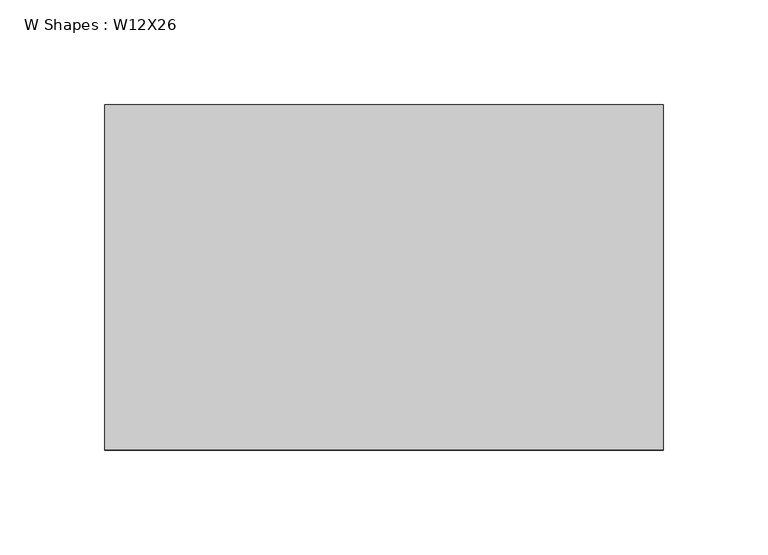
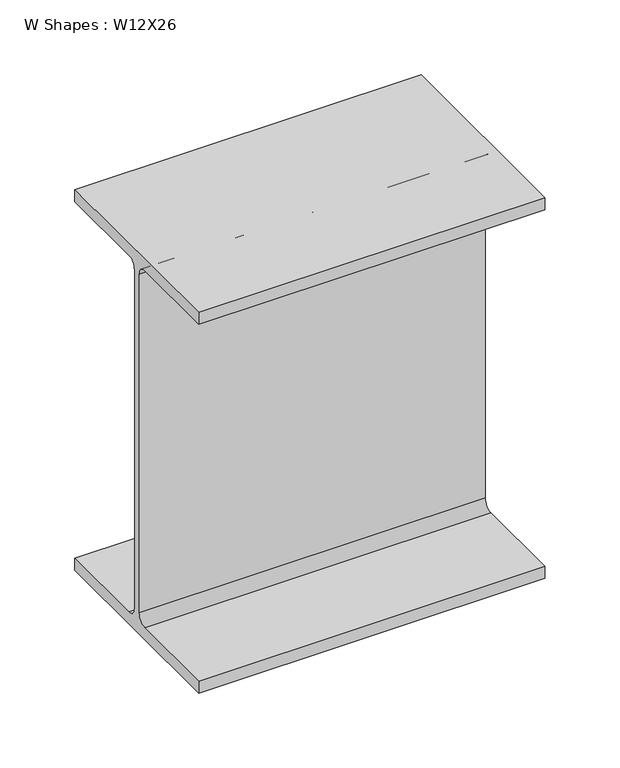
"""IFC4 building model written with IfcOpenShell, lengths in millimetres: beam geometry, W Shapes : W12X26."""

from ifc_helpers import new_model, si_unit, point, frame, frame_2d, origin, place, context, project, spatial, polyline, circle_curve, trimmed, segment, composite_curve, outline, extrude, source, transform, mapped, element, save


def w_shapes_w12x26_f1af6e5e(model_context):
    return source(origin(), model_context, "Body", "SweptSolid", [
        extrude(outline(composite_curve([segment(polyline([(82.423, -145.288), (82.423, -154.94), (-82.423, -154.94), (-82.423, -145.288), (-10.541, -145.288)]), True, "CONTINUOUS"), segment(trimmed(circle_curve(frame_2d((-10.541, -137.668)), 7.62), [point((-10.541, -145.288))], [point((-2.921, -137.668))], True, "CARTESIAN"), True, "CONTINUOUS"), segment(polyline([(-2.921, -137.668), (-2.921, 137.668)]), True, "CONTINUOUS"), segment(trimmed(circle_curve(frame_2d((-10.541, 137.668)), 7.62), [point((-2.921, 137.668))], [point((-10.541, 145.288))], True, "CARTESIAN"), True, "CONTINUOUS"), segment(polyline([(-10.541, 145.288), (-82.423, 145.288), (-82.423, 154.94), (82.423, 154.94), (82.423, 145.288), (10.541, 145.288)]), True, "CONTINUOUS"), segment(trimmed(circle_curve(frame_2d((10.541, 137.668)), 7.62), [point((10.541, 145.288))], [point((2.921, 137.668))], True, "CARTESIAN"), True, "CONTINUOUS"), segment(polyline([(2.921, 137.668), (2.921, -137.668)]), True, "CONTINUOUS"), segment(trimmed(circle_curve(frame_2d((10.541, -137.668)), 7.62), [point((2.921, -137.668))], [point((10.541, -145.288))], True, "CARTESIAN"), True, "CONTINUOUS"), segment(polyline([(10.541, -145.288), (82.423, -145.288)]), True, "CONTINUOUS")], self_intersect=False)), frame((-133.35, 0.0, 0.0), z_axis=(1.0, 0.0, 0.0), x_axis=(0.0, 1.0, 0.0)), (0.0, 0.0, 1.0), 266.7),
    ])


if __name__ == "__main__":
    model = new_model("IFC4")
    model_context = context("Model", 3, world=origin())
    ifc_project = project(units=[si_unit("LENGTHUNIT", "METRE", prefix="MILLI")], contexts=[model_context])
    site = spatial("IfcSite", under=ifc_project)
    building = spatial("IfcBuilding", under=site)
    placement = place(None, origin())
    w_shapes_w12x26_shape = w_shapes_w12x26_f1af6e5e(model_context)
    element("IfcBeam", 1, ObjectType="W Shapes : W12X26", at=placement, inside=building, context=model_context, shape_type="MappedRepresentation", body=[
        mapped(w_shapes_w12x26_shape, transform((0.0, 0.0, 0.0), x_axis=(1.0, 0.0, 0.0), y_axis=(0.0, 1.0, 0.0), z_axis=(0.0, 0.0, 1.0))),
    ])
    save(model, "model.ifc")

# Revit data of these elements
# Type "W Shapes : W12X26"
#   Section Name Key = "W12X26"
#   Assembly Code = "B10"
#   Width = 6.490"
#   Web Thickness = 0.230"
#   Web Fillet = 0.300"
#   Warping Constant = 607.00 in⁶
#   Torsional Moment of Inertia = 0.30 in⁴
#   Section Area = 7.65 in²
#   Plastic Modulus weak axis = 8.17 in³
#   Plastic Modulus strong axis = 37.20 in³
#   Perimeter = 4.116 ft²/ft
#   Nominal Weight = 26.00 lbf/ft
#   Moment of Inertia weak axis = 17.30 in⁴
#   Moment of Inertia strong axis = 204.00 in⁴
#   Height = 12.200"
#   Flange Thickness = 0.380"
#   Elastic Modulus weak axis = 5.34 in³
#   Elastic Modulus strong axis = 33.40 in³
#   Clear Web Height = 0' - 10 1/8"
#   Centroid Vertical = 6.100"
#   Centroid Horizontal = 3.245"
#   Bolt Spacing = 0' - 3 1/2"
#   Length [instance default] = 5' - 0"
#   Structural Material [instance default] = Steel ASTM A992
#   Principal Axes Angle = 0
# Element 1 (IfcBeam, "W Shapes : W12X26")
#   Materials on its faces: "Steel ASTM A992"
# Materials
#   "Steel ASTM A992": class "Metal", colour RGB 199 199 199, transparency 0, Description = "Structural steel 50ksi", Cost = 0
